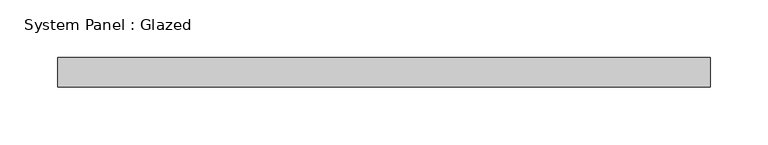
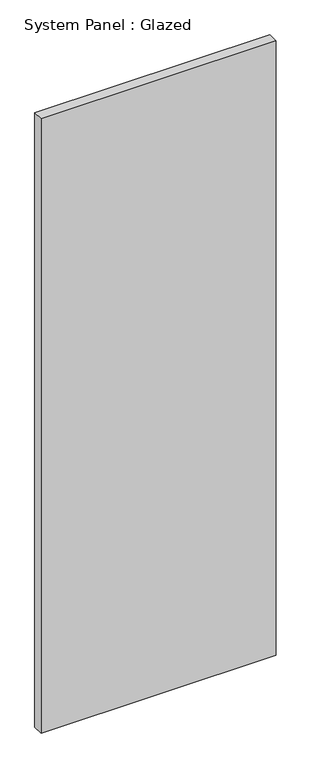
"""IFC4 building model written with IfcOpenShell, lengths in millimetres: plate geometry, System Panel : Glazed."""

from ifc_helpers import new_model, si_unit, origin, origin_with_axes, place, context, project, spatial, polyline, outline, extrude, source, transform, mapped, element, save


def system_panel_glazed_0446ff67(model_context):
    return source(origin(), model_context, "Body", "SweptSolid", [
        extrude(outline(polyline([(282.575, 19.05), (-282.575, 19.05), (-282.575, 44.45), (282.575, 44.45), (282.575, 19.05)])), origin_with_axes(), (0.0, 0.0, 1.0), 1559.2136257),
    ])


if __name__ == "__main__":
    model = new_model("IFC4")
    model_context = context("Model", 3, world=origin())
    ifc_project = project(units=[si_unit("LENGTHUNIT", "METRE", prefix="MILLI")], contexts=[model_context])
    site = spatial("IfcSite", under=ifc_project)
    building = spatial("IfcBuilding", under=site)
    placement = place(None, origin())
    system_panel_glazed_shape = system_panel_glazed_0446ff67(model_context)
    element("IfcPlate", 1, ObjectType="System Panel : Glazed", at=placement, inside=building, context=model_context, shape_type="MappedRepresentation", body=[
        mapped(system_panel_glazed_shape, transform((0.0, 0.0, 0.0), x_axis=(1.0, 0.0, 0.0), y_axis=(0.0, 1.0, 0.0), z_axis=(0.0, 0.0, 1.0))),
    ])
    save(model, "model.ifc")

# Revit data of these elements
# Type "System Panel : Glazed"
#   Construction Type Id = "GSP4R"
#   Analytic Construction = "1/8 in Pilkington single glazing"
#   Visual Light Transmittance = 0.9
#   Solar Heat Gain Coefficient = 0.86
#   Heat Transfer Coefficient (U) = 1.18115 BTU/(h·ft²·°F)
#   Define Thermal Properties by = 1
# Element 1 (IfcPlate, "System Panel : Glazed")
#   Materials on its faces: "Glass"
# Materials
#   "Glass": class "Glass", colour RGB 0 128 192, transparency 0.75, Description = "Soda Lime Glass", Cost = 0
